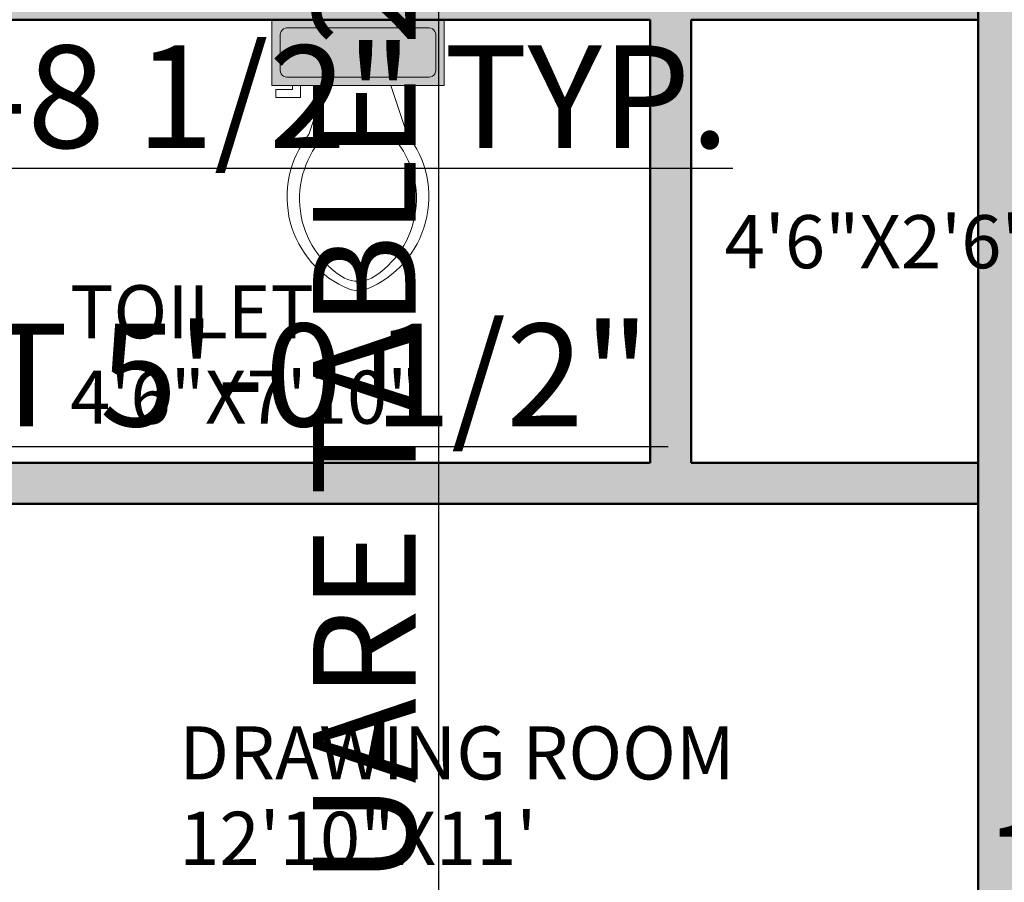
# Model space of a CAD drawing. Units: inches. Extents: x 2419 to 2878, y 1068 to 1713.
# Tile 12 of 20: x 2655 to 2775, y 1304 to 1409. Entities that reach past the tile are written whole.
import ezdxf

# ---------------------------------------------------------------- set-up
doc = ezdxf.new("R2010")
doc.units = ezdxf.units.IN
for name, color, linetype, lineweight in [('A-ANNO-DIMS', 2, 'Continuous', 18), ('A-AREA-IDEN', 7, 'Continuous', 18), ('A-FLOR-FIXT', 8, 'Continuous', 18), ('A-FLOR-PRKG-PATT', 1, 'Continuous', 13), ('A-FURN-PATT', 254, 'Continuous', 13), ('A-WALL', 7, 'Continuous', 50)]:
    doc.layers.add(name, color=color, linetype=linetype, lineweight=lineweight)
doc.layers.add('A-FLOR-FIXT-PATT', color=254, linetype='Continuous', lineweight=13, true_color=0xd7ebd2)
doc.layers.add('A-WALL-PATT', color=18, linetype='Continuous', lineweight=13, true_color=0x000000)
doc.styles.get("Standard").update_dxf_attribs({"font": 'arial.ttf'})
doc.dimstyles.new('ISO-25', dxfattribs={"dimtxt": 12.5, "dimasz": 2.5, "dimexe": 1.25, "dimexo": 0.625, "dimtad": 1, "dimdec": 0, "dimlunit": 4, "dimtxsty": 'Standard', "dimblk": 'ARCHTICK', "dimcen": 2.5, "dimse1": 1, "dimse2": 1, "dimclrd": 4, "dimadec": 0, "dimazin": 0, "dimtfac": 1, "dimtdec": 0, "dimtmove": 0, "dimatfit": 3, "dimfxl": 1, "dimarcsym": 0})

# ---------------------------------------------------------------- blocks, each defined once
blk = doc.blocks.new('*U5')
for p, q in [((9.5, -6), (9.5, -2)), ((-8, -8.5), (-8, -8)), ((-7, -8), (-7, -9.5)), ((-4, -8), (-6, -14)), ((4, -8), (6, -14)), ((-10, -8.5), (-8, -8.5)), ((-10, -9.5), (-10, -8.5)), ((-7, -9.5), (-10, -9.5)), ((4, -14), (-4, -14))]:
    blk.add_line(p, q)
blk.add_lwpolyline([(10.5, -8), (10.5, 0), (-10.5, 0), (-10.5, -8)], close=True)
for points in [[(8.5, -1), (-8.5, -1)], [(-9.5, -2), (-9.5, -6)], [(-8.5, -7), (8.5, -7)]]:
    blk.add_lwpolyline(points)
for centre, radius, start, end in [((-8.62, -1.88), 0.884, 81.8699, 188.1301), ((8.62, -1.88), 0.884, 351.8699, 98.1301), ((-8.62, -6.12), 0.884, 171.8699, 278.1301), ((8.62, -6.12), 0.884, 261.8699, 8.1301), ((3.52, -21.58), 12.17, 141.4691, 247.9714), ((4.2, -21.82), 11.33, 136.3677, 238.9468), ((-3.52, -21.58), 12.17, 292.0284, 38.5307), ((-4.2, -21.82), 11.33, 301.053, 43.6321), ((0, -27.88), 4, 245.7318, 294.2682), ((0, -29), 4, 254.8605, 285.1395)]:
    blk.add_arc(centre, radius, start, end)
blk = doc.blocks.new('_ArchTick')
at = {"color": 0, "linetype": 'ByBlock', "const_width": 0.15}
blk.add_lwpolyline([(-0.5, -0.5), (0.5, 0.5)], dxfattribs=at)
blk = doc.blocks.new('*D19')
at = {"layer": 'A-ANNO-DIMS', "color": 4, "lineweight": -2, "transparency": 16777216}
for p, q in [((2752.42, 1296.14), (2769.76, 1296.14)), ((2769.76, 1296.14), (2877.65, 1296.14))]:
    blk.add_line(p, q, dxfattribs=at)
at = {"layer": 'Defpoints', "color": 0, "transparency": 16777216}
for p in [(2769.76, 1296.14), (2752.42, 1292.99), (2769.76, 1292.99)]:
    blk.add_point(p, dxfattribs=at)
at = {"layer": 'A-ANNO-DIMS', "color": 4, "lineweight": -2, "transparency": 16777216, "xscale": 2.5, "yscale": 2.5, "zscale": 2.5, "rotation": 180}
blk.add_blockref('_ArchTick', (2752.42, 1296.14), dxfattribs=at)
at = {"layer": 'A-ANNO-DIMS', "color": 4, "lineweight": -2, "transparency": 16777216, "xscale": 2.5, "yscale": 2.5, "zscale": 2.5}
blk.add_blockref('_ArchTick', (2769.76, 1296.14), dxfattribs=at)
at = {"layer": 'A-ANNO-DIMS', "color": 0, "transparency": 16777216, "insert": (2824.95, 1303.22), "char_height": 12.5, "attachment_point": 5}
blk.add_mtext('1\'-5 1/2" TYP.', dxfattribs=at)
blk = doc.blocks.new('*D21')
at = {"layer": 'A-ANNO-DIMS', "color": 4, "lineweight": -2, "transparency": 16777216}
for p, q in [((2624.02, 1390.72), (2632.51, 1390.72)), ((2632.51, 1390.72), (2741.59, 1390.72))]:
    blk.add_line(p, q, dxfattribs=at)
at = {"layer": 'Defpoints', "color": 0, "transparency": 16777216}
for p in [(2624.02, 1392.52), (2632.51, 1392.52), (2632.51, 1390.72)]:
    blk.add_point(p, dxfattribs=at)
at = {"layer": 'A-ANNO-DIMS', "color": 4, "lineweight": -2, "transparency": 16777216, "xscale": 2.5, "yscale": 2.5, "zscale": 2.5, "rotation": 180}
blk.add_blockref('_ArchTick', (2624.02, 1390.72), dxfattribs=at)
at = {"layer": 'A-ANNO-DIMS', "color": 4, "lineweight": -2, "transparency": 16777216, "xscale": 2.5, "yscale": 2.5, "zscale": 2.5}
blk.add_blockref('_ArchTick', (2632.51, 1390.72), dxfattribs=at)
at = {"layer": 'A-ANNO-DIMS', "color": 0, "transparency": 16777216, "insert": (2688.3, 1397.81), "char_height": 12.5, "attachment_point": 5}
blk.add_mtext('0\'-8 1/2" TYP.', dxfattribs=at)
blk = doc.blocks.new('*D26')
at = {"layer": 'A-ANNO-DIMS', "color": 4, "lineweight": -2, "transparency": 16777216}
for p, q in [((2502.77, 1356.79), (2563.46, 1356.79)), ((2563.46, 1356.79), (2733.72, 1356.79))]:
    blk.add_line(p, q, dxfattribs=at)
at = {"layer": 'Defpoints', "color": 0, "transparency": 16777216}
for p in [(2563.46, 1356.79), (2502.77, 1347.69), (2563.46, 1347.69)]:
    blk.add_point(p, dxfattribs=at)
at = {"layer": 'A-ANNO-DIMS', "color": 4, "lineweight": -2, "transparency": 16777216, "xscale": 2.5, "yscale": 2.5, "zscale": 2.5, "rotation": 180}
blk.add_blockref('_ArchTick', (2502.77, 1356.79), dxfattribs=at)
at = {"layer": 'A-ANNO-DIMS', "color": 4, "lineweight": -2, "transparency": 16777216, "xscale": 2.5, "yscale": 2.5, "zscale": 2.5}
blk.add_blockref('_ArchTick', (2563.46, 1356.79), dxfattribs=at)
at = {"layer": 'A-ANNO-DIMS', "color": 0, "transparency": 16777216, "insert": (2649.84, 1363.88), "char_height": 12.5, "attachment_point": 5}
blk.add_mtext('DINING SET 5\'-0 1/2"', dxfattribs=at)
blk = doc.blocks.new('*D32')
at = {"layer": 'A-ANNO-DIMS', "color": 4, "lineweight": -2, "transparency": 16777216}
for p, q in [((2705.74, 1272.77), (2705.74, 1458.17)), ((2705.74, 1238.68), (2705.74, 1272.77))]:
    blk.add_line(p, q, dxfattribs=at)
at = {"layer": 'Defpoints', "color": 0, "transparency": 16777216}
for p in [(2705.74, 1272.77), (2710.85, 1272.77), (2710.85, 1238.68)]:
    blk.add_point(p, dxfattribs=at)
at = {"layer": 'A-ANNO-DIMS', "color": 4, "lineweight": -2, "transparency": 16777216, "xscale": 2.5, "yscale": 2.5, "zscale": 2.5}
for p, rotation in [((2705.74, 1272.77), 90), ((2705.74, 1238.68), 270)]:
    blk.add_blockref('_ArchTick', p, dxfattribs=dict(at, rotation=rotation))
at = {"layer": 'A-ANNO-DIMS', "color": 0, "transparency": 16777216, "insert": (2698.27, 1366.72), "char_height": 12.5, "attachment_point": 5, "rotation": 90}
blk.add_mtext('SQUARE TABLE 2\'-10"', dxfattribs=at)
blk = doc.blocks.new('*D36')
at = {"layer": 'A-ANNO-DIMS', "color": 4, "lineweight": -2, "transparency": 16777216}
blk.add_line((2656.74, 1605.01), (2736.32, 1605.01), dxfattribs=at)
at = {"layer": 'Defpoints', "color": 0, "transparency": 16777216}
for p in [(2736.32, 1605.01), (2656.74, 1205.81), (2736.32, 1205.81)]:
    blk.add_point(p, dxfattribs=at)
at = {"layer": 'A-ANNO-DIMS', "color": 4, "lineweight": -2, "transparency": 16777216, "xscale": 2.5, "yscale": 2.5, "zscale": 2.5, "rotation": 180}
blk.add_blockref('_ArchTick', (2656.74, 1605.01), dxfattribs=at)
at = {"layer": 'A-ANNO-DIMS', "color": 4, "lineweight": -2, "transparency": 16777216, "xscale": 2.5, "yscale": 2.5, "zscale": 2.5}
blk.add_blockref('_ArchTick', (2736.32, 1605.01), dxfattribs=at)
at = {"layer": 'A-ANNO-DIMS', "color": 0, "transparency": 16777216, "insert": (2696.53, 1612.1), "char_height": 12.5, "attachment_point": 5}
blk.add_mtext('6\'-7 1/2"', dxfattribs=at)
blk = doc.blocks.new('*D37')
at = {"layer": 'A-ANNO-DIMS', "color": 4, "lineweight": -2, "transparency": 16777216}
for p, q in [((2736.32, 1605.01), (2771.51, 1605.01)), ((2771.51, 1605.01), (2818.42, 1605.01))]:
    blk.add_line(p, q, dxfattribs=at)
at = {"layer": 'Defpoints', "color": 0, "transparency": 16777216}
for p in [(2771.51, 1605.01), (2736.32, 1205.81), (2771.51, 1205.81)]:
    blk.add_point(p, dxfattribs=at)
at = {"layer": 'A-ANNO-DIMS', "color": 4, "lineweight": -2, "transparency": 16777216, "xscale": 2.5, "yscale": 2.5, "zscale": 2.5, "rotation": 180}
blk.add_blockref('_ArchTick', (2736.32, 1605.01), dxfattribs=at)
at = {"layer": 'A-ANNO-DIMS', "color": 4, "lineweight": -2, "transparency": 16777216, "xscale": 2.5, "yscale": 2.5, "zscale": 2.5}
blk.add_blockref('_ArchTick', (2771.51, 1605.01), dxfattribs=at)
at = {"layer": 'A-ANNO-DIMS', "color": 0, "transparency": 16777216, "insert": (2796.22, 1611.91), "char_height": 12.5, "attachment_point": 5}
blk.add_mtext('2\'-11"', dxfattribs=at)
blk = doc.blocks.new('*D39')
at = {"layer": 'A-ANNO-DIMS', "color": 4, "lineweight": -2, "transparency": 16777216}
for p, q in [((2662.74, 1605.01), (2668.59, 1605.01)), ((2668.59, 1605.01), (2705.56, 1605.01))]:
    blk.add_line(p, q, dxfattribs=at)
at = {"layer": 'Defpoints', "color": 0, "transparency": 16777216}
for p in [(2668.59, 1605.01), (2662.74, 1165.6), (2668.59, 1165.6)]:
    blk.add_point(p, dxfattribs=at)
at = {"layer": 'A-ANNO-DIMS', "color": 4, "lineweight": -2, "transparency": 16777216, "xscale": 2.5, "yscale": 2.5, "zscale": 2.5, "rotation": 180}
blk.add_blockref('_ArchTick', (2662.74, 1605.01), dxfattribs=at)
at = {"layer": 'A-ANNO-DIMS', "color": 4, "lineweight": -2, "transparency": 16777216, "xscale": 2.5, "yscale": 2.5, "zscale": 2.5}
blk.add_blockref('_ArchTick', (2668.59, 1605.01), dxfattribs=at)
at = {"layer": 'A-ANNO-DIMS', "color": 0, "transparency": 16777216, "insert": (2688.32, 1612.02), "char_height": 12.5, "attachment_point": 5}
blk.add_mtext('0\'-6"', dxfattribs=at)
blk = doc.blocks.new('*D45')
at = {"layer": 'A-ANNO-DIMS', "color": 4, "lineweight": -2, "transparency": 16777216}
for p, q in [((2596.57, 1079.92), (2625.09, 1079.92)), ((2625.09, 1079.92), (2691.41, 1079.92))]:
    blk.add_line(p, q, dxfattribs=at)
at = {"layer": 'Defpoints', "color": 0, "transparency": 16777216}
for p in [(2596.57, 1408.81), (2625.09, 1408.81), (2625.09, 1079.92)]:
    blk.add_point(p, dxfattribs=at)
at = {"layer": 'A-ANNO-DIMS', "color": 4, "lineweight": -2, "transparency": 16777216, "xscale": 2.5, "yscale": 2.5, "zscale": 2.5, "rotation": 180}
blk.add_blockref('_ArchTick', (2596.57, 1079.92), dxfattribs=at)
at = {"layer": 'A-ANNO-DIMS', "color": 4, "lineweight": -2, "transparency": 16777216, "xscale": 2.5, "yscale": 2.5, "zscale": 2.5}
blk.add_blockref('_ArchTick', (2625.09, 1079.92), dxfattribs=at)
at = {"layer": 'A-ANNO-DIMS', "color": 0, "transparency": 16777216, "insert": (2659.5, 1087.01), "char_height": 12.5, "attachment_point": 5}
blk.add_mtext('2\'-4 1/2"', dxfattribs=at)
blk = doc.blocks.new('*D51')
at = {"layer": 'A-ANNO-DIMS', "color": 4, "lineweight": -2, "transparency": 16777216}
for p, q in [((2738.51, 1079.92), (2771.51, 1079.92)), ((2771.51, 1079.92), (2808.71, 1079.92))]:
    blk.add_line(p, q, dxfattribs=at)
at = {"layer": 'Defpoints', "color": 0, "transparency": 16777216}
for p in [(2738.51, 1447.89), (2771.51, 1437.39), (2771.51, 1079.92)]:
    blk.add_point(p, dxfattribs=at)
at = {"layer": 'A-ANNO-DIMS', "color": 4, "lineweight": -2, "transparency": 16777216, "xscale": 2.5, "yscale": 2.5, "zscale": 2.5, "rotation": 180}
blk.add_blockref('_ArchTick', (2738.51, 1079.92), dxfattribs=at)
at = {"layer": 'A-ANNO-DIMS', "color": 4, "lineweight": -2, "transparency": 16777216, "xscale": 2.5, "yscale": 2.5, "zscale": 2.5}
blk.add_blockref('_ArchTick', (2771.51, 1079.92), dxfattribs=at)
at = {"layer": 'A-ANNO-DIMS', "color": 0, "transparency": 16777216, "insert": (2791.36, 1086.93), "char_height": 12.5, "attachment_point": 5}
blk.add_mtext('2\'-9"', dxfattribs=at)
blk = doc.blocks.new('*D53')
at = {"layer": 'A-ANNO-DIMS', "color": 4, "lineweight": -2, "transparency": 16777216}
for p, q in [((2638.79, 1605.01), (2667.31, 1605.01)), ((2667.31, 1605.01), (2733.63, 1605.01))]:
    blk.add_line(p, q, dxfattribs=at)
at = {"layer": 'Defpoints', "color": 0, "transparency": 16777216}
for p in [(2667.31, 1605.01), (2638.79, 1217.38), (2667.31, 1217.38)]:
    blk.add_point(p, dxfattribs=at)
at = {"layer": 'A-ANNO-DIMS', "color": 4, "lineweight": -2, "transparency": 16777216, "xscale": 2.5, "yscale": 2.5, "zscale": 2.5, "rotation": 180}
blk.add_blockref('_ArchTick', (2638.79, 1605.01), dxfattribs=at)
at = {"layer": 'A-ANNO-DIMS', "color": 4, "lineweight": -2, "transparency": 16777216, "xscale": 2.5, "yscale": 2.5, "zscale": 2.5}
blk.add_blockref('_ArchTick', (2667.31, 1605.01), dxfattribs=at)
at = {"layer": 'A-ANNO-DIMS', "color": 0, "transparency": 16777216, "insert": (2701.72, 1612.1), "char_height": 12.5, "attachment_point": 5}
blk.add_mtext('2\'-4 1/2"', dxfattribs=at)
blk = doc.blocks.new('*D61')
at = {"layer": 'A-ANNO-DIMS', "color": 4, "lineweight": -2, "transparency": 16777216}
blk.add_line((2730.51, 1079.92), (2771.51, 1079.92), dxfattribs=at)
at = {"layer": 'Defpoints', "color": 0, "transparency": 16777216}
for p in [(2730.51, 1414.81), (2771.51, 1414.81), (2771.51, 1079.92)]:
    blk.add_point(p, dxfattribs=at)
at = {"layer": 'A-ANNO-DIMS', "color": 4, "lineweight": -2, "transparency": 16777216, "xscale": 2.5, "yscale": 2.5, "zscale": 2.5, "rotation": 180}
blk.add_blockref('_ArchTick', (2730.51, 1079.92), dxfattribs=at)
at = {"layer": 'A-ANNO-DIMS', "color": 4, "lineweight": -2, "transparency": 16777216, "xscale": 2.5, "yscale": 2.5, "zscale": 2.5}
blk.add_blockref('_ArchTick', (2771.51, 1079.92), dxfattribs=at)
at = {"layer": 'A-ANNO-DIMS', "color": 0, "transparency": 16777216, "insert": (2751.01, 1086.94), "char_height": 12.5, "attachment_point": 5}
blk.add_mtext('3\'-5"', dxfattribs=at)

msp = doc.modelspace()

# ---------------------------------------------------------------- hatches: boundary and pattern name
at = {"layer": 'A-FLOR-FIXT-PATT'}
h = msp.add_hatch(color=256, dxfattribs=at)
h.dxf.hatch_style = 1
h.paths.add_polyline_path([(2705.38, 1406.81, 0.5), (2704.38, 1407.81), (2687.38, 1407.81, 0.5), (2686.38, 1406.81), (2686.38, 1402.81, 0.5), (2687.38, 1401.81), (2704.38, 1401.81, 0.5), (2705.38, 1402.81)])
h.paths.add_polyline_path([(2770.51, 1456.39, 0.5), (2769.51, 1457.39), (2765.51, 1457.39, 0.5), (2764.51, 1456.39), (2764.51, 1439.39, 0.5), (2765.51, 1438.39), (2769.51, 1438.39, 0.5), (2770.51, 1439.39)])
h.paths.add_polyline_path([(2641.68, 1567.61), (2662.48, 1567.61), (2662.48, 1554.41), (2664.88, 1554.41), (2664.88, 1567.61), (2685.68, 1567.61), (2685.68, 1552.41), (2680.48, 1552.41), (2693.68, 1539.21), (2693.68, 1568.81), (2633.68, 1568.81), (2633.68, 1554.41), (2641.68, 1554.41)])
h.paths.add_polyline_path([(2678.48, 1554.41), (2678.48, 1539.21), (2693.68, 1539.21)], flags=17)
h = msp.add_hatch(color=256, dxfattribs=at)
h.dxf.hatch_style = 1
h.paths.add_polyline_path([(2771.51, 1458.39), (2763.51, 1458.39), (2763.51, 1437.39), (2771.51, 1437.39)])
h.paths.add_polyline_path([(2770.51, 1456.39, 0.5), (2769.51, 1457.39), (2765.51, 1457.39, 0.5), (2764.51, 1456.39), (2764.51, 1439.39, 0.5), (2765.51, 1438.39), (2769.51, 1438.39, 0.5), (2770.51, 1439.39)], flags=16)
h.paths.add_polyline_path([(2706.38, 1408.81), (2685.38, 1408.81), (2685.38, 1400.81), (2706.38, 1400.81)])
h.paths.add_polyline_path([(2704.38, 1401.81, 0.5), (2705.38, 1402.81), (2705.38, 1406.81, 0.5), (2704.38, 1407.81), (2687.38, 1407.81, 0.5), (2686.38, 1406.81), (2686.38, 1402.81, 0.5), (2687.38, 1401.81)], flags=16)
h.paths.add_polyline_path([(2574.48, 1207.45), (2633.94, 1207.45), (2633.94, 1217.37), (2574.48, 1217.37)], flags=9)
h.paths.add_polyline_path([(2574.45, 1217.83), (2610.47, 1217.83), (2610.47, 1227.88), (2574.45, 1227.88)], flags=9)
h.paths.add_polyline_path([(2672.43, 1304.02), (2718.62, 1304.02), (2718.62, 1313.94), (2672.43, 1313.94)], flags=9)
h.paths.add_polyline_path([(2672.4, 1314.4), (2750.13, 1314.4), (2750.13, 1324.45), (2672.4, 1324.45)], flags=9)
h.paths.add_polyline_path([(2500.43, 1374.44), (2544.8, 1374.44), (2544.8, 1384.36), (2500.43, 1384.36)], flags=9)
h.paths.add_polyline_path([(2500.41, 1384.82), (2566.08, 1384.82), (2566.08, 1394.87), (2500.41, 1394.87)], flags=9)
h.paths.add_polyline_path([(2738.93, 1376.75), (2778.27, 1376.75), (2778.27, 1386.67), (2738.93, 1386.67)], flags=9)
h.paths.add_polyline_path([(2659.12, 1357.8), (2703.49, 1357.8), (2703.49, 1367.72), (2659.12, 1367.72)], flags=9)
h.paths.add_polyline_path([(2659.1, 1368.18), (2694.11, 1368.18), (2694.11, 1378.23), (2659.1, 1378.23)], flags=9)
h.paths.add_polyline_path([(2730.12, 1466.07), (2769.46, 1466.07), (2769.46, 1475.99), (2730.12, 1475.99)], flags=9)
h.paths.add_polyline_path([(2730.1, 1476.45), (2765.12, 1476.45), (2765.12, 1486.5), (2730.1, 1486.5)], flags=9)
h.paths.add_polyline_path([(2730.38, 1518.65), (2761.48, 1518.65), (2761.48, 1528.57), (2730.38, 1528.57)], flags=9)
h.paths.add_polyline_path([(2730.36, 1529.03), (2780.96, 1529.03), (2780.96, 1539.07), (2730.36, 1539.07)], flags=9)
h.paths.add_polyline_path([(2629.32, 1455.19), (2688.78, 1455.19), (2688.78, 1465.11), (2629.32, 1465.11)], flags=9)
h.paths.add_polyline_path([(2629.3, 1465.57), (2681.9, 1465.57), (2681.9, 1475.62), (2629.3, 1475.62)], flags=9)
h.paths.add_polyline_path([(2513.23, 1456.48), (2562.63, 1456.48), (2562.63, 1466.4), (2513.23, 1466.4)], flags=9)
h.paths.add_polyline_path([(2513.21, 1466.86), (2556.26, 1466.86), (2556.26, 1476.91), (2513.21, 1476.91)], flags=9)
h.paths.add_polyline_path([(2488.87, 1521.54), (2519.97, 1521.54), (2519.97, 1531.46), (2488.87, 1531.46)], flags=9)
h.paths.add_polyline_path([(2536.55, 1543.51), (2580.92, 1543.51), (2580.92, 1553.43), (2536.55, 1553.43)], flags=9)
h.paths.add_polyline_path([(2536.56, 1553.92), (2573.53, 1553.92), (2573.53, 1563.8), (2536.56, 1563.8)], flags=9)
at = {"layer": 'A-FLOR-PRKG-PATT'}
h = msp.add_hatch(color=256, dxfattribs=at)
h.dxf.hatch_style = 1
edge = h.paths.add_edge_path()
edge.add_ellipse((2561.37, 1279.45), major_axis=(3.99, 0), ratio=0.842304, start_angle=0.6466, end_angle=90)
edge.add_line((2561.37, 1282.81), (2511.57, 1282.81))
edge.add_ellipse((2511.57, 1279.45), major_axis=(3.99, 0), ratio=0.842304, start_angle=90, end_angle=179.3534)
edge.add_ellipse((10560.89, 1188.62), major_axis=(-8054.03, 0), ratio=0.8423039, start_angle=-0.646554, end_angle=-0.628237)
edge.add_ellipse((2509.23, 1276.91), major_axis=(1.69, 0), ratio=0.842304, start_angle=179.3718, end_angle=248.4648)
edge.add_ellipse((10560.33, 1188.62), major_axis=(8052.29, 0), ratio=0.8423039, start_angle=179.353446, end_angle=179.381357, ccw=False)
edge.add_ellipse((2511.01, 1279.45), major_axis=(2.25, 0), ratio=0.842304, start_angle=90, end_angle=179.3534, ccw=False)
edge.add_line((2511.01, 1281.35), (2561.94, 1281.35))
edge.add_ellipse((2561.94, 1279.45), major_axis=(-2.25, 0), ratio=0.842304, start_angle=180.6466, end_angle=270, ccw=False)
edge.add_ellipse((-5487.38, 1188.62), major_axis=(8052.29, 0), ratio=0.8423039, start_angle=0.528271, end_angle=0.646554, ccw=False)
edge.add_ellipse((2563.71, 1276.91), major_axis=(-1.69, 0), ratio=0.842304, start_angle=111.5352, end_angle=180.6282)
edge.add_ellipse((-5487.95, 1188.62), major_axis=(-8054.03, 0), ratio=0.8423039, start_angle=180.628237, end_angle=180.646554)
edge = h.paths.add_edge_path()
edge.add_ellipse((2564.91, 1261.91), major_axis=(-1.12, 0), ratio=0.842304, start_angle=180, end_angle=270)
edge.add_line((2564.91, 1262.86), (2564.43, 1262.86))
edge.add_ellipse((-5487.38, 1188.62), major_axis=(8052.29, 0), ratio=0.8423039, start_angle=0.383867, end_angle=0.528271, ccw=False)
edge.add_line((2564.65, 1242.56), (2564.91, 1242.56))
edge.add_ellipse((2564.91, 1243.51), major_axis=(-1.12, 0), ratio=0.842304, start_angle=90, end_angle=180)
edge.add_line((2566.03, 1243.51), (2566.03, 1261.91))
edge = h.paths.add_edge_path()
edge.add_ellipse((2564.91, 1174.99), major_axis=(1.12, 0), ratio=0.842304, start_angle=0, end_angle=90)
edge.add_line((2564.91, 1175.94), (2564.89, 1175.94))
edge.add_ellipse((-5487.38, 1188.62), major_axis=(8052.29, 0), ratio=0.8423039, start_angle=-0.134987, end_angle=-0.090229, ccw=False)
edge.add_ellipse((2163.34, 1170.91), major_axis=(401.54, 0), ratio=0.842304, start_angle=-2.18, end_angle=-0.1356, ccw=False)
edge.add_line((2564.47, 1155.64), (2564.91, 1155.64))
edge.add_ellipse((2564.91, 1156.59), major_axis=(-1.12, 0), ratio=0.842304, start_angle=90, end_angle=180)
edge.add_line((2566.03, 1156.59), (2566.03, 1174.99))
h.paths.add_polyline_path([(2574.48, 1207.45), (2633.94, 1207.45), (2633.94, 1217.37), (2574.48, 1217.37)], flags=9)
h.paths.add_polyline_path([(2574.45, 1217.83), (2610.47, 1217.83), (2610.47, 1227.88), (2574.45, 1227.88)], flags=9)
h.paths.add_polyline_path([(2672.43, 1304.02), (2718.62, 1304.02), (2718.62, 1313.94), (2672.43, 1313.94)], flags=9)
h.paths.add_polyline_path([(2672.4, 1314.4), (2750.13, 1314.4), (2750.13, 1324.45), (2672.4, 1324.45)], flags=9)
h.paths.add_polyline_path([(2500.43, 1374.44), (2544.8, 1374.44), (2544.8, 1384.36), (2500.43, 1384.36)], flags=9)
h.paths.add_polyline_path([(2500.41, 1384.82), (2566.08, 1384.82), (2566.08, 1394.87), (2500.41, 1394.87)], flags=9)
h.paths.add_polyline_path([(2738.93, 1376.75), (2778.27, 1376.75), (2778.27, 1386.67), (2738.93, 1386.67)], flags=9)
h.paths.add_polyline_path([(2659.12, 1357.8), (2703.49, 1357.8), (2703.49, 1367.72), (2659.12, 1367.72)], flags=9)
h.paths.add_polyline_path([(2659.1, 1368.18), (2694.11, 1368.18), (2694.11, 1378.23), (2659.1, 1378.23)], flags=9)
h.paths.add_polyline_path([(2730.12, 1466.07), (2769.46, 1466.07), (2769.46, 1475.99), (2730.12, 1475.99)], flags=9)
h.paths.add_polyline_path([(2730.1, 1476.45), (2765.12, 1476.45), (2765.12, 1486.5), (2730.1, 1486.5)], flags=9)
h.paths.add_polyline_path([(2730.38, 1518.65), (2761.48, 1518.65), (2761.48, 1528.57), (2730.38, 1528.57)], flags=9)
h.paths.add_polyline_path([(2730.36, 1529.03), (2780.96, 1529.03), (2780.96, 1539.07), (2730.36, 1539.07)], flags=9)
h.paths.add_polyline_path([(2629.32, 1455.19), (2688.78, 1455.19), (2688.78, 1465.11), (2629.32, 1465.11)], flags=9)
h.paths.add_polyline_path([(2629.3, 1465.57), (2681.9, 1465.57), (2681.9, 1475.62), (2629.3, 1475.62)], flags=9)
h.paths.add_polyline_path([(2513.23, 1456.48), (2562.63, 1456.48), (2562.63, 1466.4), (2513.23, 1466.4)], flags=9)
h.paths.add_polyline_path([(2513.21, 1466.86), (2556.26, 1466.86), (2556.26, 1476.91), (2513.21, 1476.91)], flags=9)
h.paths.add_polyline_path([(2488.87, 1521.54), (2519.97, 1521.54), (2519.97, 1531.46), (2488.87, 1531.46)], flags=9)
h.paths.add_polyline_path([(2536.55, 1543.51), (2580.92, 1543.51), (2580.92, 1553.43), (2536.55, 1553.43)], flags=9)
h.paths.add_polyline_path([(2536.56, 1553.92), (2573.53, 1553.92), (2573.53, 1563.8), (2536.56, 1563.8)], flags=9)
at = {"layer": 'A-FURN-PATT'}
h = msp.add_hatch(color=256, dxfattribs=at)
h.dxf.hatch_style = 1
h.paths.add_polyline_path([(2710.17, 1562.64), (2707.17, 1559.64), (2709.17, 1559.64, -0.414214), (2710.17, 1560.64)])
h.paths.add_polyline_path([(2711.17, 1559.64, 1), (2709.17, 1559.64, 1)])
h.paths.add_polyline_path([(2710.17, 1562.64), (2710.17, 1560.64, -0.414214), (2711.17, 1559.64), (2713.17, 1559.64)])
h.paths.add_polyline_path([(2713.17, 1559.64), (2711.17, 1559.64, -0.414214), (2710.17, 1558.64), (2710.17, 1556.64)])
h.paths.add_polyline_path([(2710.17, 1558.64, -0.414214), (2709.17, 1559.64), (2707.17, 1559.64), (2710.17, 1556.64)])
h.paths.add_polyline_path([(2613.13, 1558.89, 1), (2611.13, 1558.89, 1)])
h.paths.add_polyline_path([(2612.13, 1561.89), (2612.13, 1559.89, -0.414214), (2613.13, 1558.89), (2615.13, 1558.89)])
h.paths.add_polyline_path([(2612.13, 1559.89), (2612.13, 1561.89), (2609.13, 1558.89), (2611.13, 1558.89, -0.414214)])
h.paths.add_polyline_path([(2612.13, 1557.89, -0.414214), (2611.13, 1558.89), (2609.13, 1558.89), (2612.13, 1555.89)])
h.paths.add_polyline_path([(2574.48, 1207.45), (2633.94, 1207.45), (2633.94, 1217.37), (2574.48, 1217.37)], flags=9)
h.paths.add_polyline_path([(2574.45, 1217.83), (2610.47, 1217.83), (2610.47, 1227.88), (2574.45, 1227.88)], flags=9)
h.paths.add_polyline_path([(2672.43, 1304.02), (2718.62, 1304.02), (2718.62, 1313.94), (2672.43, 1313.94)], flags=9)
h.paths.add_polyline_path([(2672.4, 1314.4), (2750.13, 1314.4), (2750.13, 1324.45), (2672.4, 1324.45)], flags=9)
h.paths.add_polyline_path([(2500.43, 1374.44), (2544.8, 1374.44), (2544.8, 1384.36), (2500.43, 1384.36)], flags=9)
h.paths.add_polyline_path([(2500.41, 1384.82), (2566.08, 1384.82), (2566.08, 1394.87), (2500.41, 1394.87)], flags=9)
h.paths.add_polyline_path([(2738.93, 1376.75), (2778.27, 1376.75), (2778.27, 1386.67), (2738.93, 1386.67)], flags=9)
h.paths.add_polyline_path([(2659.12, 1357.8), (2703.49, 1357.8), (2703.49, 1367.72), (2659.12, 1367.72)], flags=9)
h.paths.add_polyline_path([(2659.1, 1368.18), (2694.11, 1368.18), (2694.11, 1378.23), (2659.1, 1378.23)], flags=9)
h.paths.add_polyline_path([(2730.12, 1466.07), (2769.46, 1466.07), (2769.46, 1475.99), (2730.12, 1475.99)], flags=9)
h.paths.add_polyline_path([(2730.1, 1476.45), (2765.12, 1476.45), (2765.12, 1486.5), (2730.1, 1486.5)], flags=9)
h.paths.add_polyline_path([(2730.38, 1518.65), (2761.48, 1518.65), (2761.48, 1528.57), (2730.38, 1528.57)], flags=9)
h.paths.add_polyline_path([(2730.36, 1529.03), (2780.96, 1529.03), (2780.96, 1539.07), (2730.36, 1539.07)], flags=9)
h.paths.add_polyline_path([(2629.32, 1455.19), (2688.78, 1455.19), (2688.78, 1465.11), (2629.32, 1465.11)], flags=9)
h.paths.add_polyline_path([(2629.3, 1465.57), (2681.9, 1465.57), (2681.9, 1475.62), (2629.3, 1475.62)], flags=9)
h.paths.add_polyline_path([(2513.23, 1456.48), (2562.63, 1456.48), (2562.63, 1466.4), (2513.23, 1466.4)], flags=9)
h.paths.add_polyline_path([(2513.21, 1466.86), (2556.26, 1466.86), (2556.26, 1476.91), (2513.21, 1476.91)], flags=9)
h.paths.add_polyline_path([(2488.87, 1521.54), (2519.97, 1521.54), (2519.97, 1531.46), (2488.87, 1531.46)], flags=9)
h.paths.add_polyline_path([(2536.55, 1543.51), (2580.92, 1543.51), (2580.92, 1553.43), (2536.55, 1553.43)], flags=9)
h.paths.add_polyline_path([(2536.56, 1553.92), (2573.53, 1553.92), (2573.53, 1563.8), (2536.56, 1563.8)], flags=9)
at = {"layer": 'A-WALL-PATT'}
h = msp.add_hatch(color=256, dxfattribs=at)
h.dxf.hatch_style = 1
h.paths.add_polyline_path([(2780.51, 1577.81), (2471.51, 1577.81), (2471.51, 1121.81), (2780.51, 1121.81)])
h.paths.add_polyline_path([(2480.51, 1568.81), (2771.51, 1568.81), (2771.51, 1130.81), (2480.51, 1130.81)], flags=16)
h.paths.add_polyline_path([(2528.51, 1568.81), (2528.51, 1512.81), (2594.51, 1512.81), (2594.51, 1414.81), (2596.57, 1414.81), (2596.57, 1441.61), (2597.82, 1441.61), (2597.82, 1441.58, -0.384016), (2625.03, 1414.81), (2725.51, 1414.81), (2725.51, 1567.55), (2728.3, 1567.55), (2746.89, 1567.55), (2746.89, 1566.73), (2746.87, 1566.73, -0.367216), (2730.51, 1549.09), (2730.51, 1512.81), (2750.85, 1512.81), (2750.85, 1510.03, -0.401453), (2733.08, 1491.46), (2733.08, 1491.44), (2732.27, 1491.44), (2732.27, 1507.81), (2730.51, 1507.81), (2730.51, 1408.81), (2736.51, 1408.81), (2736.51, 1349.81), (2632.51, 1349.81), (2632.51, 1408.81), (2528.51, 1408.81), (2528.51, 1414.81), (2503.97, 1414.81), (2503.97, 1494.85), (2558.38, 1494.85), (2558.38, 1507.81), (2529.96, 1507.81, -0.414214), (2530.82, 1506.96), (2530.82, 1497.26, -0.414214), (2529.96, 1496.4), (2514.56, 1496.4, -0.414214), (2513.7, 1497.26), (2513.7, 1506.96, -0.414214), (2514.56, 1507.81), (2528.51, 1507.81), (2528.51, 1512.81), (2480.51, 1512.81)], flags=0)
h.paths.add_polyline_path([(2516.26, 1507.81), (2528.26, 1507.81), (2528.26, 1505.81), (2523.42, 1505.81), (2524.07, 1504.67), (2529.39, 1504.67, -0.414214), (2529.96, 1504.1), (2529.96, 1497.83, -0.414214), (2529.39, 1497.26), (2515.13, 1497.26, -0.414214), (2514.56, 1497.83), (2514.56, 1504.1, -0.414214), (2515.13, 1504.67), (2520.69, 1504.67), (2521.34, 1505.81), (2516.26, 1505.81)], flags=0)
h.paths.add_polyline_path([(2522.02, 1505.53), (2522.82, 1507.32, -0.65506), (2522.25, 1506.06), (2522.19, 1505.93), (2522.43, 1505.53)], flags=0)
h.paths.add_polyline_path([(2522.83, 1500.97, -1), (2521.69, 1500.97, -1)], flags=0)
h.paths.add_polyline_path([(2522.55, 1500.97, -1), (2521.98, 1500.97, -1)], flags=0)
h.paths.add_polyline_path([(2482.01, 1470.63), (2499.89, 1470.63), (2499.89, 1448.27), (2482.01, 1448.27), (2482.01, 1452.74), (2481.26, 1452.74), (2481.26, 1449.76), (2480.51, 1449.76), (2480.51, 1469.14), (2481.26, 1469.14), (2481.26, 1466.16), (2482.01, 1466.16)], flags=0)
h.paths.add_polyline_path([(2488.71, 1466.16, -1), (2484.24, 1466.16, -1)], flags=0)
h.paths.add_polyline_path([(2496.17, 1466.16, -1), (2490.2, 1466.16, -1)], flags=0)
h.paths.add_polyline_path([(2487.97, 1466.16, -1), (2484.99, 1466.16, -1)], flags=0)
h.paths.add_polyline_path([(2495.42, 1466.16, -1), (2490.95, 1466.16, -1)], flags=0)
h.paths.add_polyline_path([(2487.22, 1466.16, -1), (2485.73, 1466.16, -1)], flags=0)
h.paths.add_polyline_path([(2494.68, 1466.16, -1), (2491.69, 1466.16, -1)], flags=0)
h.paths.add_polyline_path([(2499.11, 1468, -1), (2497.98, 1468, -1)], flags=0)
h.paths.add_polyline_path([(2493.93, 1466.16, -1), (2492.44, 1466.16, -1)], flags=0)
h.paths.add_polyline_path([(2499.37, 1463.71, -1), (2498.17, 1463.71, -1)], flags=0)
h.paths.add_polyline_path([(2484.24, 1461.69), (2496.17, 1461.69), (2496.17, 1457.22), (2484.24, 1457.22)], flags=0)
h.paths.add_polyline_path([(2484.99, 1460.94), (2495.42, 1460.94), (2495.42, 1457.96), (2484.99, 1457.96)], flags=0)
h.paths.add_polyline_path([(2586.88, 1510.03), (2587.69, 1510.03), (2587.69, 1491.44), (2586.88, 1491.44)], flags=0)
h.paths.add_polyline_path([(2499.26, 1459.41, -1), (2498.2, 1459.41, -1)], flags=0)
h.paths.add_polyline_path([(2489.46, 1452.74, -1), (2483.5, 1452.74, -1)], flags=0)
h.paths.add_polyline_path([(2557.3, 1408.81), (2557.3, 1413.09, -0.401453), (2584.57, 1441.58), (2584.57, 1441.61), (2585.82, 1441.61), (2585.82, 1413.09), (2585.82, 1408.81)], flags=0)
h.paths.add_polyline_path([(2488.71, 1452.74, -1), (2484.24, 1452.74, -1)], flags=0)
h.paths.add_polyline_path([(2495.42, 1452.74, -1), (2490.95, 1452.74, -1)], flags=0)
h.paths.add_polyline_path([(2487.97, 1452.74, -1), (2484.99, 1452.74, -1)], flags=0)
h.paths.add_polyline_path([(2494.68, 1452.74, -1), (2491.69, 1452.74, -1)], flags=0)
h.paths.add_polyline_path([(2487.22, 1452.74, -1), (2485.73, 1452.74, -1)], flags=0)
h.paths.add_polyline_path([(2499.18, 1454.44, -1), (2497.9, 1454.44, -1)], flags=0)
h.paths.add_polyline_path([(2493.93, 1452.74, -1), (2492.44, 1452.74, -1)], flags=0)
h.paths.add_polyline_path([(2499.3, 1450.64, -1), (2497.79, 1450.64, -1)], flags=0)
h.paths.add_polyline_path([(2619.13, 1558.89, -1), (2605.13, 1558.89, -1)], flags=0)
h.paths.add_polyline_path([(2609.13, 1558.89), (2612.13, 1561.89), (2615.13, 1558.89), (2612.13, 1555.89)], flags=0)
h.paths.add_polyline_path([(2611.13, 1558.89, -1), (2613.13, 1558.89, -1)], flags=0)
h.paths.add_polyline_path([(2633.68, 1568.81), (2693.68, 1568.81), (2693.68, 1488.81), (2633.68, 1488.81)], flags=0)
h.paths.add_polyline_path([(2641.68, 1554.41), (2641.68, 1567.61), (2662.48, 1567.61), (2662.48, 1554.41), (2664.88, 1554.41), (2664.88, 1567.61), (2685.68, 1567.61), (2685.68, 1552.41), (2680.48, 1552.41), (2693.68, 1539.21), (2678.48, 1539.21), (2678.48, 1554.41)], flags=0)
h.paths.add_polyline_path([(2637.51, 1408.81), (2731.51, 1408.81), (2731.51, 1354.81), (2637.51, 1354.81), (2637.51, 1357.98), (2635.3, 1357.98), (2635.3, 1358.79), (2637.51, 1358.79)], flags=0)
h.paths.add_polyline_path([(2717.17, 1559.64, -1), (2703.17, 1559.64, -1)], flags=0)
h.paths.add_polyline_path([(2707.17, 1559.64), (2710.17, 1562.64), (2713.17, 1559.64), (2710.17, 1556.64)], flags=0)
h.paths.add_polyline_path([(2709.17, 1559.64, -1), (2711.17, 1559.64, -1)], flags=0)
h.paths.add_polyline_path([(2685.38, 1408.81), (2706.38, 1408.81), (2706.38, 1400.81), (2699.88, 1400.81), (2701.88, 1394.81, -0.501323), (2696.92, 1375.95, -0.132891), (2694.83, 1375.95, -0.501317), (2689.88, 1394.81), (2691.88, 1400.81), (2688.88, 1400.81), (2688.88, 1399.31), (2685.88, 1399.31), (2685.88, 1400.31), (2687.88, 1400.31), (2687.88, 1400.81), (2685.38, 1400.81)], flags=0)
h.paths.add_polyline_path([(2687.38, 1407.81), (2704.38, 1407.81, -0.5), (2705.38, 1406.81), (2705.38, 1402.81, -0.5), (2704.38, 1401.81), (2687.38, 1401.81, -0.5), (2686.38, 1402.81), (2686.38, 1406.81, -0.5)], flags=0)
h.paths.add_polyline_path([(2639.51, 1205.81), (2634.51, 1205.81), (2634.51, 1293.81), (2637.51, 1293.81), (2639.51, 1293.81)], flags=0)
h.paths.add_polyline_path([(2691.88, 1394.81), (2699.88, 1394.81, -0.48008), (2697.52, 1377.29, -0.215004), (2694.23, 1377.29, -0.48008)], flags=0)
h.paths.add_polyline_path([(2757.51, 1453.89), (2763.51, 1451.89), (2763.51, 1454.89), (2762.01, 1454.89), (2762.01, 1457.89), (2763.01, 1457.89), (2763.01, 1455.89), (2763.51, 1455.89), (2763.51, 1458.39), (2771.51, 1458.39), (2771.51, 1437.39), (2763.51, 1437.39), (2763.51, 1443.89), (2757.51, 1441.89, -0.501323), (2738.65, 1446.85, -0.132891), (2738.65, 1448.94, -0.501317)], flags=0)
h.paths.add_polyline_path([(2739.99, 1449.54, -0.48008), (2757.51, 1451.89), (2757.51, 1443.89, -0.48008), (2739.99, 1446.25, -0.215004)], flags=0)
h.paths.add_polyline_path([(2765.51, 1457.39), (2769.51, 1457.39, -0.5), (2770.51, 1456.39), (2770.51, 1439.39, -0.5), (2769.51, 1438.39), (2765.51, 1438.39, -0.5), (2764.51, 1439.39), (2764.51, 1456.39, -0.5)], flags=0)
h = msp.add_hatch(color=256, dxfattribs=at)
h.dxf.hatch_style = 1
h.paths.add_polyline_path([(2771.51, 1354.81), (2736.51, 1354.81), (2736.51, 1408.81), (2771.51, 1408.81), (2771.51, 1414.81), (2625.03, 1414.81, -0.015108), (2625.09, 1413.09), (2625.09, 1408.81), (2632.51, 1408.81), (2632.51, 1376.56), (2635.3, 1376.56, -0.029838), (2637.51, 1376.43), (2637.51, 1408.81), (2731.51, 1408.81), (2731.51, 1354.81), (2637.51, 1354.81), (2637.51, 1357.98), (2635.3, 1357.98), (2632.51, 1357.98), (2632.51, 1349.81), (2771.51, 1349.81)])
h.paths.add_polyline_path([(2639.51, 1298.81), (2637.51, 1298.81), (2480.51, 1298.81), (2480.51, 1293.81), (2637.51, 1293.81), (2639.51, 1293.81)])
h.paths.add_polyline_path([(2639.51, 1293.81), (2637.51, 1293.81), (2634.51, 1293.81), (2634.51, 1244.65), (2638.79, 1244.65, -0.006332), (2639.51, 1244.64)])
h.paths.add_polyline_path([(2639.51, 1205.81), (2771.51, 1205.81), (2771.51, 1210.81), (2639.51, 1210.81), (2639.51, 1216.13), (2638.79, 1216.13), (2634.51, 1216.13), (2634.51, 1130.81), (2639.51, 1130.81)])
h.paths.add_polyline_path([(2596.57, 1413.09), (2596.57, 1414.81), (2585.82, 1414.81), (2585.82, 1413.09), (2585.82, 1408.81), (2596.57, 1408.81)])
h.paths.add_polyline_path([(2557.3, 1413.09, -0.015108), (2557.35, 1414.81), (2480.51, 1414.81), (2480.51, 1408.81), (2557.3, 1408.81)])
h.paths.add_polyline_path([(2574.48, 1207.45), (2633.94, 1207.45), (2633.94, 1217.37), (2574.48, 1217.37)], flags=9)
h.paths.add_polyline_path([(2574.45, 1217.83), (2610.47, 1217.83), (2610.47, 1227.88), (2574.45, 1227.88)], flags=9)
h.paths.add_polyline_path([(2672.43, 1304.02), (2718.62, 1304.02), (2718.62, 1313.94), (2672.43, 1313.94)], flags=9)
h.paths.add_polyline_path([(2672.4, 1314.4), (2750.13, 1314.4), (2750.13, 1324.45), (2672.4, 1324.45)], flags=9)
h.paths.add_polyline_path([(2500.43, 1374.44), (2544.8, 1374.44), (2544.8, 1384.36), (2500.43, 1384.36)], flags=9)
h.paths.add_polyline_path([(2500.41, 1384.82), (2566.08, 1384.82), (2566.08, 1394.87), (2500.41, 1394.87)], flags=9)
h.paths.add_polyline_path([(2738.93, 1376.75), (2778.27, 1376.75), (2778.27, 1386.67), (2738.93, 1386.67)], flags=9)
h.paths.add_polyline_path([(2659.12, 1357.8), (2703.49, 1357.8), (2703.49, 1367.72), (2659.12, 1367.72)], flags=25)
h.paths.add_polyline_path([(2659.1, 1368.18), (2694.11, 1368.18), (2694.11, 1378.23), (2659.1, 1378.23)], flags=25)
h.paths.add_polyline_path([(2730.12, 1466.07), (2769.46, 1466.07), (2769.46, 1475.99), (2730.12, 1475.99)], flags=9)
h.paths.add_polyline_path([(2730.1, 1476.45), (2765.12, 1476.45), (2765.12, 1486.5), (2730.1, 1486.5)], flags=9)
h.paths.add_polyline_path([(2730.38, 1518.65), (2761.48, 1518.65), (2761.48, 1528.57), (2730.38, 1528.57)], flags=9)
h.paths.add_polyline_path([(2730.36, 1529.03), (2780.96, 1529.03), (2780.96, 1539.07), (2730.36, 1539.07)], flags=9)
h.paths.add_polyline_path([(2629.32, 1455.19), (2688.78, 1455.19), (2688.78, 1465.11), (2629.32, 1465.11)], flags=9)
h.paths.add_polyline_path([(2629.3, 1465.57), (2681.9, 1465.57), (2681.9, 1475.62), (2629.3, 1475.62)], flags=9)
h.paths.add_polyline_path([(2513.23, 1456.48), (2562.63, 1456.48), (2562.63, 1466.4), (2513.23, 1466.4)], flags=9)
h.paths.add_polyline_path([(2513.21, 1466.86), (2556.26, 1466.86), (2556.26, 1476.91), (2513.21, 1476.91)], flags=9)
h.paths.add_polyline_path([(2488.87, 1521.54), (2519.97, 1521.54), (2519.97, 1531.46), (2488.87, 1531.46)], flags=9)
h.paths.add_polyline_path([(2536.55, 1543.51), (2580.92, 1543.51), (2580.92, 1553.43), (2536.55, 1553.43)], flags=9)
h.paths.add_polyline_path([(2536.56, 1553.92), (2573.53, 1553.92), (2573.53, 1563.8), (2536.56, 1563.8)], flags=9)

# ---------------------------------------------------------------- linework, layer by layer
at = {"layer": 'A-WALL'}
for p, q in [((2771.51, 1568.81), (2771.51, 1130.81)), ((2637.51, 1408.81), (2731.51, 1408.81)), ((2637.51, 1408.81), (2731.51, 1408.81)), ((2731.51, 1354.81), (2731.51, 1408.81)), ((2736.51, 1354.81), (2736.51, 1408.81)), ((2736.51, 1408.81), (2771.51, 1408.81)), ((2736.51, 1408.81), (2771.51, 1408.81)), ((2637.51, 1354.81), (2731.51, 1354.81)), ((2736.51, 1354.81), (2771.51, 1354.81)), ((2632.51, 1349.81), (2771.51, 1349.81))]:
    msp.add_line(p, q, dxfattribs=at)

# ---------------------------------------------------------------- block references
at = {"layer": 'A-FLOR-FIXT'}
msp.add_blockref('*U5', (2695.88, 1408.81), dxfattribs=at)

# ---------------------------------------------------------------- texts
at = {"layer": 'A-AREA-IDEN'}
for s, height, p in [('4\'6"X2\'6"', 6.475, (2740.59, 1378.51)), ('TOILET', 6.475, (2660.77, 1369.97)), ('4\'6"X7\'10"', 6.475, (2660.77, 1359.56)), ('DRAWING ROOM', 6.4753, (2674.08, 1316.19)), ('12\'10"X11\'', 6.475, (2674.08, 1305.78))]:
    msp.add_text(s, height=height, dxfattribs=at).set_placement(p)

# ---------------------------------------------------------------- dimensions: what is measured, and where the dimension line sits
at = {"layer": 'A-ANNO-DIMS'}
for base, p1, p2, picture, middle in [((2667.31, 1605.01), (2638.79, 1217.38), (2667.31, 1217.38), '*D53', (2701.72, 1612.1)), ((2736.32, 1605.01), (2656.74, 1205.81), (2736.32, 1205.81), '*D36', (2696.53, 1612.1)), ((2668.5856, 1605.013), (2662.7408, 1165.6026), (2668.5856, 1165.6026), '*D39', (2688.3247, 1612.0201)), ((2771.51, 1605.01), (2736.32, 1205.81), (2771.51, 1205.81), '*D37', (2796.22, 1611.91)), ((2771.51, 1079.92), (2738.51, 1447.89), (2771.51, 1437.39), '*D51', (2791.36, 1086.93)), ((2771.51, 1079.92), (2730.51, 1414.81), (2771.51, 1414.81), '*D61', (2751.01, 1086.94)), ((2625.09, 1079.92), (2596.57, 1408.81), (2625.09, 1408.81), '*D45', (2659.5, 1087.01))]:
    dim = msp.add_linear_dim(base=base, p1=p1, p2=p2, dimstyle='ISO-25', override={"dimdec": 1, "dimlfac": 1, "dimrnd": 0, "dimzin": 1, "dimdsep": 46, "dimlunit": 4, "dimfrac": 2}, dxfattribs=at)
    dim.commit()
    dim.dimension.update_dxf_attribs({"geometry": picture, "text_midpoint": middle})
dim = msp.add_linear_dim(base=(2705.74, 1272.77), p1=(2710.85, 1238.68), p2=(2710.85, 1272.77), angle=90, text='SQUARE TABLE <>', dimstyle='ISO-25', override={"dimdec": 1, "dimlfac": 1, "dimrnd": 0, "dimzin": 1, "dimdsep": 46, "dimlunit": 4, "dimfrac": 2}, dxfattribs=at)
dim.commit()
dim.dimension.update_dxf_attribs({"geometry": '*D32', "text_midpoint": (2698.27, 1366.72)})
for base, p1, p2, text, picture, middle in [((2632.51, 1390.72), (2624.02, 1392.52), (2632.51, 1392.52), '<> TYP.', '*D21', (2688.3, 1397.81)), ((2563.46, 1356.79), (2502.77, 1347.69), (2563.46, 1347.69), 'DINING SET <>', '*D26', (2649.84, 1363.88)), ((2769.76, 1296.14), (2752.42, 1292.99), (2769.76, 1292.99), '<> TYP.', '*D19', (2824.95, 1303.22))]:
    dim = msp.add_linear_dim(base=base, p1=p1, p2=p2, text=text, dimstyle='ISO-25', override={"dimdec": 1, "dimlfac": 1, "dimrnd": 0, "dimzin": 1, "dimdsep": 46, "dimlunit": 4, "dimfrac": 2}, dxfattribs=at)
    dim.commit()
    dim.dimension.update_dxf_attribs({"geometry": picture, "text_midpoint": middle})

doc.saveas('drawing.dxf')
